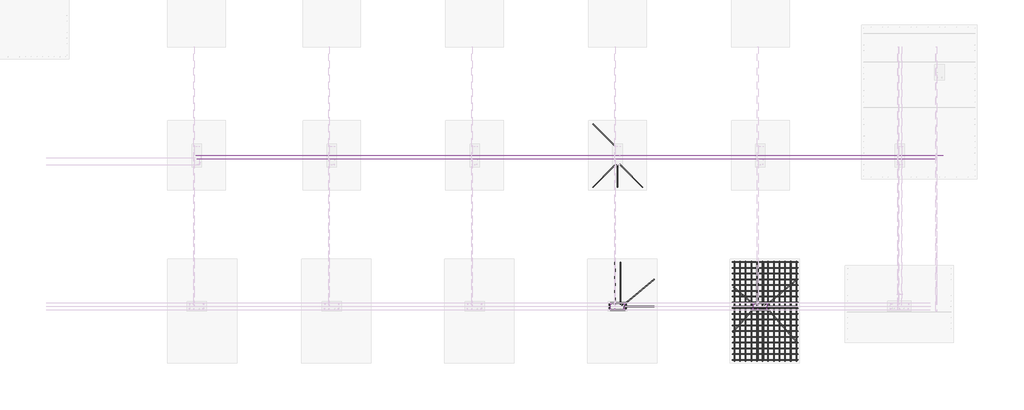
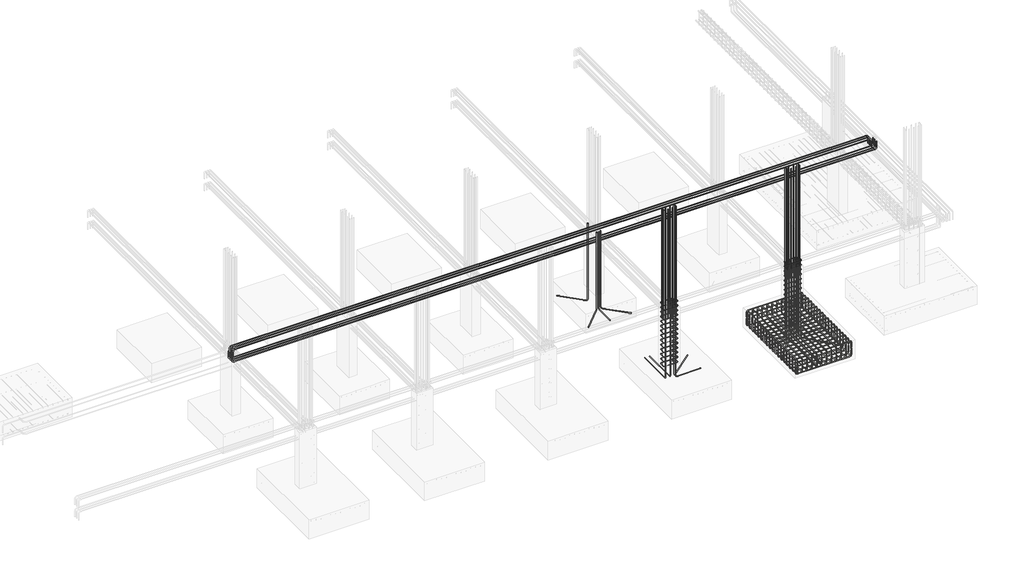
# One storey, part 7 of 18: 39 reinforcing bars.
"""IFC4 building model written with IfcOpenShell, lengths in millimetres."""

from ifc_helpers import new_model, si_unit, point, frame, origin, place, context, project, spatial, polyline, circle_curve, trimmed, segment, composite_curve, source, transform, mapped, element, save
from ifc_brep_helpers import swept_disk

model = new_model("IFC4")

# Units and contexts
model_context = context("Model", 3, world=origin())
ifc_project = project(units=[si_unit("LENGTHUNIT", "METRE", prefix="MILLI")], contexts=[model_context])

# Site, building, storey
site = spatial("IfcSite", under=ifc_project)
building = spatial("IfcBuilding", under=site)
storey = spatial("IfcBuildingStorey", under=building, Elevation=-2000.0)

# Reinforcing bars
placement = place(None, origin())
reinforcing_bar_shape = source(origin(), model_context, "Body", "SolidModel", [
    swept_disk(composite_curve([segment(polyline([(6891.7059943, -4415.5752408, -2300.0), (6891.7059943, -4415.5752408, -2486.6)]), True, "CONTINUOUS"), segment(trimmed(circle_curve(frame((6836.2559943, -4415.5752408, -2486.6), z_axis=(0.0, 1.0, 0.0), x_axis=(55.45000000000073, 0.0, 0.0)), 55.45), [point((6891.7059943, -4415.5752408, -2486.6))], [point((6836.2559943, -4415.5752408, -2542.05))], True, "CARTESIAN"), True, "CONTINUOUS"), segment(polyline([(6836.2559943, -4415.5752408, -2542.05), (5263.0559943, -4415.5752408, -2542.05)]), True, "CONTINUOUS"), segment(trimmed(circle_curve(frame((5263.0559943, -4415.5752408, -2486.6), z_axis=(0.0, 1.0, 0.0), x_axis=(0.0, 0.0, -55.45000000000027)), 55.45), [point((5263.0559943, -4415.5752408, -2542.05))], [point((5207.6059943, -4415.5752408, -2486.6))], True, "CARTESIAN"), True, "CONTINUOUS"), segment(polyline([(5207.6059943, -4415.5752408, -2486.6), (5207.6059943, -4415.5752408, -2300.0)]), True, "CONTINUOUS")], self_intersect=False), 7.95),
])
element("IfcReinforcingBar", 1, at=placement, inside=storey, context=model_context, shape_type="MappedRepresentation", body=[
    mapped(reinforcing_bar_shape, transform((0.0, 0.0, 0.0), x_axis=(1.0, 0.0, 0.0), y_axis=(0.0, 1.0, 0.0), z_axis=(0.0, 0.0, 1.0))),
    mapped(reinforcing_bar_shape, transform((0.0, -148.9809282, 0.0), x_axis=(1.0, 0.0, 0.0), y_axis=(0.0, 1.0, 0.0), z_axis=(0.0, 0.0, 1.0))),
    mapped(reinforcing_bar_shape, transform((0.0, -297.9618564, 0.0), x_axis=(1.0, 0.0, 0.0), y_axis=(0.0, 1.0, 0.0), z_axis=(0.0, 0.0, 1.0))),
    mapped(reinforcing_bar_shape, transform((0.0, -446.9427846, 0.0), x_axis=(1.0, 0.0, 0.0), y_axis=(0.0, 1.0, 0.0), z_axis=(0.0, 0.0, 1.0))),
    mapped(reinforcing_bar_shape, transform((0.0, -595.9237129, 0.0), x_axis=(1.0, 0.0, 0.0), y_axis=(0.0, 1.0, 0.0), z_axis=(0.0, 0.0, 1.0))),
    mapped(reinforcing_bar_shape, transform((0.0, -744.9046411, 0.0), x_axis=(1.0, 0.0, 0.0), y_axis=(0.0, 1.0, 0.0), z_axis=(0.0, 0.0, 1.0))),
    mapped(reinforcing_bar_shape, transform((0.0, -893.8855693, 0.0), x_axis=(1.0, 0.0, 0.0), y_axis=(0.0, 1.0, 0.0), z_axis=(0.0, 0.0, 1.0))),
    mapped(reinforcing_bar_shape, transform((0.0, -1042.8664975, 0.0), x_axis=(1.0, 0.0, 0.0), y_axis=(0.0, 1.0, 0.0), z_axis=(0.0, 0.0, 1.0))),
    mapped(reinforcing_bar_shape, transform((0.0, -1191.8474257, 0.0), x_axis=(1.0, 0.0, 0.0), y_axis=(0.0, 1.0, 0.0), z_axis=(0.0, 0.0, 1.0))),
    mapped(reinforcing_bar_shape, transform((0.0, -1340.8283539, 0.0), x_axis=(1.0, 0.0, 0.0), y_axis=(0.0, 1.0, 0.0), z_axis=(0.0, 0.0, 1.0))),
    mapped(reinforcing_bar_shape, transform((0.0, -1489.8092821, 0.0), x_axis=(1.0, 0.0, 0.0), y_axis=(0.0, 1.0, 0.0), z_axis=(0.0, 0.0, 1.0))),
    mapped(reinforcing_bar_shape, transform((0.0, -1638.7902103, 0.0), x_axis=(1.0, 0.0, 0.0), y_axis=(0.0, 1.0, 0.0), z_axis=(0.0, 0.0, 1.0))),
    mapped(reinforcing_bar_shape, transform((0.0, -1787.7711386, 0.0), x_axis=(1.0, 0.0, 0.0), y_axis=(0.0, 1.0, 0.0), z_axis=(0.0, 0.0, 1.0))),
    mapped(reinforcing_bar_shape, transform((0.0, -1936.7520668, 0.0), x_axis=(1.0, 0.0, 0.0), y_axis=(0.0, 1.0, 0.0), z_axis=(0.0, 0.0, 1.0))),
    mapped(reinforcing_bar_shape, transform((0.0, -2085.732995, 0.0), x_axis=(1.0, 0.0, 0.0), y_axis=(0.0, 1.0, 0.0), z_axis=(0.0, 0.0, 1.0))),
    mapped(reinforcing_bar_shape, transform((0.0, -2234.7139232, 0.0), x_axis=(1.0, 0.0, 0.0), y_axis=(0.0, 1.0, 0.0), z_axis=(0.0, 0.0, 1.0))),
    mapped(reinforcing_bar_shape, transform((0.0, -2383.6948514, 0.0), x_axis=(1.0, 0.0, 0.0), y_axis=(0.0, 1.0, 0.0), z_axis=(0.0, 0.0, 1.0))),
    mapped(reinforcing_bar_shape, transform((0.0, -2532.6757796, 0.0), x_axis=(1.0, 0.0, 0.0), y_axis=(0.0, 1.0, 0.0), z_axis=(0.0, 0.0, 1.0))),
])
reinforcing_bar_2_shape = source(origin(), model_context, "Body", "SolidModel", [
    swept_disk(composite_curve([segment(polyline([(5205.6559943, -4415.5752408, -2250.0), (5205.6559943, -4415.5752408, -2102.0)]), True, "CONTINUOUS"), segment(trimmed(circle_curve(frame((5251.6559943, -4415.5752408, -2102.0), z_axis=(0.0, 1.0, 0.0), x_axis=(-46.0, 0.0, 0.0)), 46.0), [point((5205.6559943, -4415.5752408, -2102.0))], [point((5251.6559943, -4415.5752408, -2056.0))], True, "CARTESIAN"), True, "CONTINUOUS"), segment(polyline([(5251.6559943, -4415.5752408, -2056.0), (6847.6559943, -4415.5752408, -2056.0)]), True, "CONTINUOUS"), segment(trimmed(circle_curve(frame((6847.6559943, -4415.5752408, -2102.0), z_axis=(0.0, 1.0, 0.0), x_axis=(0.0, 0.0, 46.0)), 46.0), [point((6847.6559943, -4415.5752408, -2056.0))], [point((6893.6559943, -4415.5752408, -2102.0))], True, "CARTESIAN"), True, "CONTINUOUS"), segment(polyline([(6893.6559943, -4415.5752408, -2102.0), (6893.6559943, -4415.5752408, -2250.0)]), True, "CONTINUOUS")], self_intersect=False), 6.0),
])
element("IfcReinforcingBar", 2, at=placement, inside=storey, context=model_context, shape_type="MappedRepresentation", body=[
    mapped(reinforcing_bar_2_shape, transform((0.0, 0.0, 0.0), x_axis=(1.0, 0.0, 0.0), y_axis=(0.0, 1.0, 0.0), z_axis=(0.0, 0.0, 1.0))),
    mapped(reinforcing_bar_2_shape, transform((0.0, -148.9809282, 0.0), x_axis=(1.0, 0.0, 0.0), y_axis=(0.0, 1.0, 0.0), z_axis=(0.0, 0.0, 1.0))),
    mapped(reinforcing_bar_2_shape, transform((0.0, -297.9618564, 0.0), x_axis=(1.0, 0.0, 0.0), y_axis=(0.0, 1.0, 0.0), z_axis=(0.0, 0.0, 1.0))),
    mapped(reinforcing_bar_2_shape, transform((0.0, -446.9427846, 0.0), x_axis=(1.0, 0.0, 0.0), y_axis=(0.0, 1.0, 0.0), z_axis=(0.0, 0.0, 1.0))),
    mapped(reinforcing_bar_2_shape, transform((0.0, -595.9237129, 0.0), x_axis=(1.0, 0.0, 0.0), y_axis=(0.0, 1.0, 0.0), z_axis=(0.0, 0.0, 1.0))),
    mapped(reinforcing_bar_2_shape, transform((0.0, -744.9046411, 0.0), x_axis=(1.0, 0.0, 0.0), y_axis=(0.0, 1.0, 0.0), z_axis=(0.0, 0.0, 1.0))),
    mapped(reinforcing_bar_2_shape, transform((0.0, -893.8855693, 0.0), x_axis=(1.0, 0.0, 0.0), y_axis=(0.0, 1.0, 0.0), z_axis=(0.0, 0.0, 1.0))),
    mapped(reinforcing_bar_2_shape, transform((0.0, -1042.8664975, 0.0), x_axis=(1.0, 0.0, 0.0), y_axis=(0.0, 1.0, 0.0), z_axis=(0.0, 0.0, 1.0))),
    mapped(reinforcing_bar_2_shape, transform((0.0, -1191.8474257, 0.0), x_axis=(1.0, 0.0, 0.0), y_axis=(0.0, 1.0, 0.0), z_axis=(0.0, 0.0, 1.0))),
    mapped(reinforcing_bar_2_shape, transform((0.0, -1340.8283539, 0.0), x_axis=(1.0, 0.0, 0.0), y_axis=(0.0, 1.0, 0.0), z_axis=(0.0, 0.0, 1.0))),
    mapped(reinforcing_bar_2_shape, transform((0.0, -1489.8092821, 0.0), x_axis=(1.0, 0.0, 0.0), y_axis=(0.0, 1.0, 0.0), z_axis=(0.0, 0.0, 1.0))),
    mapped(reinforcing_bar_2_shape, transform((0.0, -1638.7902103, 0.0), x_axis=(1.0, 0.0, 0.0), y_axis=(0.0, 1.0, 0.0), z_axis=(0.0, 0.0, 1.0))),
    mapped(reinforcing_bar_2_shape, transform((0.0, -1787.7711386, 0.0), x_axis=(1.0, 0.0, 0.0), y_axis=(0.0, 1.0, 0.0), z_axis=(0.0, 0.0, 1.0))),
    mapped(reinforcing_bar_2_shape, transform((0.0, -1936.7520668, 0.0), x_axis=(1.0, 0.0, 0.0), y_axis=(0.0, 1.0, 0.0), z_axis=(0.0, 0.0, 1.0))),
    mapped(reinforcing_bar_2_shape, transform((0.0, -2085.732995, 0.0), x_axis=(1.0, 0.0, 0.0), y_axis=(0.0, 1.0, 0.0), z_axis=(0.0, 0.0, 1.0))),
    mapped(reinforcing_bar_2_shape, transform((0.0, -2234.7139232, 0.0), x_axis=(1.0, 0.0, 0.0), y_axis=(0.0, 1.0, 0.0), z_axis=(0.0, 0.0, 1.0))),
    mapped(reinforcing_bar_2_shape, transform((0.0, -2383.6948514, 0.0), x_axis=(1.0, 0.0, 0.0), y_axis=(0.0, 1.0, 0.0), z_axis=(0.0, 0.0, 1.0))),
    mapped(reinforcing_bar_2_shape, transform((0.0, -2532.6757796, 0.0), x_axis=(1.0, 0.0, 0.0), y_axis=(0.0, 1.0, 0.0), z_axis=(0.0, 0.0, 1.0))),
])
reinforcing_bar_3_shape = source(origin(), model_context, "Body", "SolidModel", [
    swept_disk(composite_curve([segment(polyline([(5251.8367771, -4392.6797656, -2322.6684255), (5251.8367771, -4392.6797656, -2470.6684255)]), True, "CONTINUOUS"), segment(trimmed(circle_curve(frame((5251.8367771, -4438.6797656, -2470.6684255), z_axis=(-1.0, 0.0, 0.0), x_axis=(0.0, 46.0, 0.0)), 46.0), [point((5251.8367771, -4392.6797656, -2470.6684255))], [point((5251.8367771, -4438.6797656, -2516.6684255))], True, "CARTESIAN"), True, "CONTINUOUS"), segment(polyline([(5251.8367771, -4438.6797656, -2516.6684255), (5251.8367771, -6934.6797656, -2516.6684255)]), True, "CONTINUOUS"), segment(trimmed(circle_curve(frame((5251.8367771, -6934.6797656, -2470.6684255), z_axis=(-1.0, 0.0, 0.0), x_axis=(0.0, 0.0, -46.0)), 46.0), [point((5251.8367771, -6934.6797656, -2516.6684255))], [point((5251.8367771, -6980.6797656, -2470.6684255))], True, "CARTESIAN"), True, "CONTINUOUS"), segment(polyline([(5251.8367771, -6980.6797656, -2470.6684255), (5251.8367771, -6980.6797656, -2322.6684255)]), True, "CONTINUOUS")], self_intersect=False), 6.0),
])
element("IfcReinforcingBar", 3, at=placement, inside=storey, context=model_context, shape_type="MappedRepresentation", body=[
    mapped(reinforcing_bar_3_shape, transform((0.0, 0.0, 0.0), x_axis=(1.0, 0.0, 0.0), y_axis=(0.0, 1.0, 0.0), z_axis=(0.0, 0.0, 1.0))),
    mapped(reinforcing_bar_3_shape, transform((145.8017329, 0.0, 0.0), x_axis=(1.0, 0.0, 0.0), y_axis=(0.0, 1.0, 0.0), z_axis=(0.0, 0.0, 1.0))),
    mapped(reinforcing_bar_3_shape, transform((291.6034659, 0.0, 0.0), x_axis=(1.0, 0.0, 0.0), y_axis=(0.0, 1.0, 0.0), z_axis=(0.0, 0.0, 1.0))),
    mapped(reinforcing_bar_3_shape, transform((437.4051988, 0.0, 0.0), x_axis=(1.0, 0.0, 0.0), y_axis=(0.0, 1.0, 0.0), z_axis=(0.0, 0.0, 1.0))),
    mapped(reinforcing_bar_3_shape, transform((583.2069318, 0.0, 0.0), x_axis=(1.0, 0.0, 0.0), y_axis=(0.0, 1.0, 0.0), z_axis=(0.0, 0.0, 1.0))),
    mapped(reinforcing_bar_3_shape, transform((729.0086647, 0.0, 0.0), x_axis=(1.0, 0.0, 0.0), y_axis=(0.0, 1.0, 0.0), z_axis=(0.0, 0.0, 1.0))),
    mapped(reinforcing_bar_3_shape, transform((874.8103976, 0.0, 0.0), x_axis=(1.0, 0.0, 0.0), y_axis=(0.0, 1.0, 0.0), z_axis=(0.0, 0.0, 1.0))),
    mapped(reinforcing_bar_3_shape, transform((1020.6121306, 0.0, 0.0), x_axis=(1.0, 0.0, 0.0), y_axis=(0.0, 1.0, 0.0), z_axis=(0.0, 0.0, 1.0))),
    mapped(reinforcing_bar_3_shape, transform((1166.4138635, 0.0, 0.0), x_axis=(1.0, 0.0, 0.0), y_axis=(0.0, 1.0, 0.0), z_axis=(0.0, 0.0, 1.0))),
    mapped(reinforcing_bar_3_shape, transform((1312.2155965, 0.0, 0.0), x_axis=(1.0, 0.0, 0.0), y_axis=(0.0, 1.0, 0.0), z_axis=(0.0, 0.0, 1.0))),
    mapped(reinforcing_bar_3_shape, transform((1458.0173294, 0.0, 0.0), x_axis=(1.0, 0.0, 0.0), y_axis=(0.0, 1.0, 0.0), z_axis=(0.0, 0.0, 1.0))),
    mapped(reinforcing_bar_3_shape, transform((1603.8190623, 0.0, 0.0), x_axis=(1.0, 0.0, 0.0), y_axis=(0.0, 1.0, 0.0), z_axis=(0.0, 0.0, 1.0))),
])
reinforcing_bar_4_shape = source(origin(), model_context, "Body", "SolidModel", [
    swept_disk(composite_curve([segment(polyline([(6857.5790113, -4392.6797656, -2276.6677805), (6857.5790113, -4392.6797656, -2128.6677805)]), True, "CONTINUOUS"), segment(trimmed(circle_curve(frame((6857.5790113, -4438.6797656, -2128.6677805), z_axis=(1.0, 0.0, 0.0), x_axis=(0.0, 46.0, 0.0)), 46.0), [point((6857.5790113, -4392.6797656, -2128.6677805))], [point((6857.5790113, -4438.6797656, -2082.6677805))], True, "CARTESIAN"), True, "CONTINUOUS"), segment(polyline([(6857.5790113, -4438.6797656, -2082.6677805), (6857.5790113, -6934.6797656, -2082.6677805)]), True, "CONTINUOUS"), segment(trimmed(circle_curve(frame((6857.5790113, -6934.6797656, -2128.6677805), z_axis=(1.0, 0.0, 0.0), x_axis=(0.0, 0.0, 46.0)), 46.0), [point((6857.5790113, -6934.6797656, -2082.6677805))], [point((6857.5790113, -6980.6797656, -2128.6677805))], True, "CARTESIAN"), True, "CONTINUOUS"), segment(polyline([(6857.5790113, -6980.6797656, -2128.6677805), (6857.5790113, -6980.6797656, -2276.6677805)]), True, "CONTINUOUS")], self_intersect=False), 6.0),
])
element("IfcReinforcingBar", 4, at=placement, inside=storey, context=model_context, shape_type="MappedRepresentation", body=[
    mapped(reinforcing_bar_4_shape, transform((0.0, 0.0, 0.0), x_axis=(1.0, 0.0, 0.0), y_axis=(0.0, 1.0, 0.0), z_axis=(0.0, 0.0, 1.0))),
    mapped(reinforcing_bar_4_shape, transform((-145.9765667, 0.0, 0.0), x_axis=(1.0, 0.0, 0.0), y_axis=(0.0, 1.0, 0.0), z_axis=(0.0, 0.0, 1.0))),
    mapped(reinforcing_bar_4_shape, transform((-291.9531335, 0.0, 0.0), x_axis=(1.0, 0.0, 0.0), y_axis=(0.0, 1.0, 0.0), z_axis=(0.0, 0.0, 1.0))),
    mapped(reinforcing_bar_4_shape, transform((-437.9297002, 0.0, 0.0), x_axis=(1.0, 0.0, 0.0), y_axis=(0.0, 1.0, 0.0), z_axis=(0.0, 0.0, 1.0))),
    mapped(reinforcing_bar_4_shape, transform((-583.906267, 0.0, 0.0), x_axis=(1.0, 0.0, 0.0), y_axis=(0.0, 1.0, 0.0), z_axis=(0.0, 0.0, 1.0))),
    mapped(reinforcing_bar_4_shape, transform((-729.8828337, 0.0, 0.0), x_axis=(1.0, 0.0, 0.0), y_axis=(0.0, 1.0, 0.0), z_axis=(0.0, 0.0, 1.0))),
    mapped(reinforcing_bar_4_shape, transform((-875.8594005, 0.0, 0.0), x_axis=(1.0, 0.0, 0.0), y_axis=(0.0, 1.0, 0.0), z_axis=(0.0, 0.0, 1.0))),
    mapped(reinforcing_bar_4_shape, transform((-1021.8359672, 0.0, 0.0), x_axis=(1.0, 0.0, 0.0), y_axis=(0.0, 1.0, 0.0), z_axis=(0.0, 0.0, 1.0))),
    mapped(reinforcing_bar_4_shape, transform((-1167.8125339, 0.0, 0.0), x_axis=(1.0, 0.0, 0.0), y_axis=(0.0, 1.0, 0.0), z_axis=(0.0, 0.0, 1.0))),
    mapped(reinforcing_bar_4_shape, transform((-1313.7891007, 0.0, 0.0), x_axis=(1.0, 0.0, 0.0), y_axis=(0.0, 1.0, 0.0), z_axis=(0.0, 0.0, 1.0))),
    mapped(reinforcing_bar_4_shape, transform((-1459.7656674, 0.0, 0.0), x_axis=(1.0, 0.0, 0.0), y_axis=(0.0, 1.0, 0.0), z_axis=(0.0, 0.0, 1.0))),
    mapped(reinforcing_bar_4_shape, transform((-1605.7422342, 0.0, 0.0), x_axis=(1.0, 0.0, 0.0), y_axis=(0.0, 1.0, 0.0), z_axis=(0.0, 0.0, 1.0))),
])
reinforcing_bar_5_shape = source(origin(), model_context, "Body", "SolidModel", [
    swept_disk(composite_curve([segment(polyline([(6039.5684825, -5535.5091206, -34.0), (6095.9039341, -5479.1736689, -34.0)]), True, "CONTINUOUS"), segment(trimmed(circle_curve(frame((6116.4100308, -5499.6797656, -34.0), z_axis=(0.0, 0.0, -1.0), x_axis=(-20.506096699999944, 20.506096699999944, 0.0)), 29.0), [point((6095.9039341, -5479.1736689, -34.0))], [point((6145.4100308, -5499.6797656, -34.0))], True, "CARTESIAN"), True, "CONTINUOUS"), segment(polyline([(6145.4100308, -5499.6797656, -34.0), (6145.4100308, -5623.6797656, -34.0)]), True, "CONTINUOUS"), segment(trimmed(circle_curve(frame((6116.4100308, -5623.6797656, -34.0), z_axis=(0.0, 0.0, -1.0), x_axis=(29.0, 0.0, 0.0)), 29.0), [point((6145.4100308, -5623.6797656, -34.0))], [point((6116.4100308, -5652.6797656, -34.0))], True, "CARTESIAN"), True, "CONTINUOUS"), segment(polyline([(6116.4100308, -5652.6797656, -34.0), (5742.4100308, -5652.6797656, -34.0)]), True, "CONTINUOUS"), segment(trimmed(circle_curve(frame((5742.4100308, -5623.707741, -32.7265044), z_axis=(0.0, 0.043913640913297095, -0.9990353307775146), x_axis=(0.0, -28.972024599999713, -1.2734955999999968)), 29.0), [point((5742.4100308, -5652.6797656, -34.0))], [point((5713.4100308, -5623.707741, -32.7265044))], True, "CARTESIAN"), True, "CONTINUOUS"), segment(polyline([(5713.4100308, -5623.707741, -32.7265044), (5713.4100308, -5499.6517902, -27.2734956)]), True, "CONTINUOUS"), segment(trimmed(circle_curve(frame((5742.4100308, -5499.6517902, -27.2734956), z_axis=(0.0, 0.043913640913297095, -0.9990353307775146), x_axis=(-29.0, 0.0, 0.0)), 29.0), [point((5713.4100308, -5499.6517902, -27.2734956))], [point((5742.4100308, -5470.6797656, -26.0))], True, "CARTESIAN"), True, "CONTINUOUS"), segment(polyline([(5742.4100308, -5470.6797656, -26.0), (6116.4100308, -5470.6797656, -26.0)]), True, "CONTINUOUS"), segment(trimmed(circle_curve(frame((6116.4100308, -5499.6797656, -26.0), z_axis=(0.0, 0.0, -1.0), x_axis=(0.0, 29.0, 0.0)), 29.0), [point((6116.4100308, -5470.6797656, -26.0))], [point((6136.9161274, -5520.1858622, -26.0))], True, "CARTESIAN"), True, "CONTINUOUS"), segment(polyline([(6136.9161274, -5520.1858622, -26.0), (6080.5806758, -5576.5213139, -26.0)]), True, "CONTINUOUS")], self_intersect=False), 4.0),
])
element("IfcReinforcingBar", 5, at=placement, inside=storey, context=model_context, shape_type="MappedRepresentation", body=[
    mapped(reinforcing_bar_5_shape, transform((0.0, 0.0, 0.0), x_axis=(1.0, 0.0, 0.0), y_axis=(0.0, 1.0, 0.0), z_axis=(0.0, 0.0, 1.0))),
    mapped(reinforcing_bar_5_shape, transform((0.0, 0.0, -148.6153846), x_axis=(1.0, 0.0, 0.0), y_axis=(0.0, 1.0, 0.0), z_axis=(0.0, 0.0, 1.0))),
    mapped(reinforcing_bar_5_shape, transform((0.0, 0.0, -297.2307692), x_axis=(1.0, 0.0, 0.0), y_axis=(0.0, 1.0, 0.0), z_axis=(0.0, 0.0, 1.0))),
    mapped(reinforcing_bar_5_shape, transform((0.0, 0.0, -445.8461538), x_axis=(1.0, 0.0, 0.0), y_axis=(0.0, 1.0, 0.0), z_axis=(0.0, 0.0, 1.0))),
    mapped(reinforcing_bar_5_shape, transform((0.0, 0.0, -594.4615385), x_axis=(1.0, 0.0, 0.0), y_axis=(0.0, 1.0, 0.0), z_axis=(0.0, 0.0, 1.0))),
    mapped(reinforcing_bar_5_shape, transform((0.0, 0.0, -743.0769231), x_axis=(1.0, 0.0, 0.0), y_axis=(0.0, 1.0, 0.0), z_axis=(0.0, 0.0, 1.0))),
    mapped(reinforcing_bar_5_shape, transform((0.0, 0.0, -891.6923077), x_axis=(1.0, 0.0, 0.0), y_axis=(0.0, 1.0, 0.0), z_axis=(0.0, 0.0, 1.0))),
    mapped(reinforcing_bar_5_shape, transform((0.0, 0.0, -1040.3076923), x_axis=(1.0, 0.0, 0.0), y_axis=(0.0, 1.0, 0.0), z_axis=(0.0, 0.0, 1.0))),
    mapped(reinforcing_bar_5_shape, transform((0.0, 0.0, -1188.9230769), x_axis=(1.0, 0.0, 0.0), y_axis=(0.0, 1.0, 0.0), z_axis=(0.0, 0.0, 1.0))),
    mapped(reinforcing_bar_5_shape, transform((0.0, 0.0, -1337.5384615), x_axis=(1.0, 0.0, 0.0), y_axis=(0.0, 1.0, 0.0), z_axis=(0.0, 0.0, 1.0))),
    mapped(reinforcing_bar_5_shape, transform((0.0, 0.0, -1486.1538462), x_axis=(1.0, 0.0, 0.0), y_axis=(0.0, 1.0, 0.0), z_axis=(0.0, 0.0, 1.0))),
    mapped(reinforcing_bar_5_shape, transform((0.0, 0.0, -1634.7692308), x_axis=(1.0, 0.0, 0.0), y_axis=(0.0, 1.0, 0.0), z_axis=(0.0, 0.0, 1.0))),
    mapped(reinforcing_bar_5_shape, transform((0.0, 0.0, -1783.3846154), x_axis=(1.0, 0.0, 0.0), y_axis=(0.0, 1.0, 0.0), z_axis=(0.0, 0.0, 1.0))),
    mapped(reinforcing_bar_5_shape, transform((0.0, 0.0, -1932.0), x_axis=(1.0, 0.0, 0.0), y_axis=(0.0, 1.0, 0.0), z_axis=(0.0, 0.0, 1.0))),
])
element("IfcReinforcingBar", 6, at=placement, inside=storey, context=model_context, shape_type="SolidModel", body=[
    swept_disk(composite_curve([segment(polyline([(5226.3766571, -5063.6864072, -2480.0), (5699.5441951, -5460.7211138, -2480.0)]), True, "CONTINUOUS"), segment(trimmed(circle_curve(frame((5699.5441951, -5460.7211138, -2412.5), z_axis=(-0.6427876096865429, -0.7660444431189751, 0.0), x_axis=(0.0, 0.0, -67.5)), 67.5), [point((5699.5441951, -5460.7211138, -2480.0))], [point((5751.252195, -5504.1092774, -2412.5))], True, "CARTESIAN"), True, "CONTINUOUS"), segment(polyline([(5751.252195, -5504.1092774, -2412.5), (5751.252195, -5504.1092774, -20.0)]), True, "CONTINUOUS")], self_intersect=False), 10.0),
])
element("IfcReinforcingBar", 7, at=placement, inside=storey, context=model_context, shape_type="SolidModel", body=[
    swept_disk(composite_curve([segment(polyline([(5222.3423379, -5559.3632831, -2480.0), (5694.892069, -5559.3632831, -2480.0)]), True, "CONTINUOUS"), segment(trimmed(circle_curve(frame((5694.892069, -5559.3632831, -2434.0), z_axis=(0.0, -1.0, 0.0), x_axis=(0.0, 0.0, -46.0)), 46.0), [point((5694.892069, -5559.3632831, -2480.0))], [point((5740.892069, -5559.3632831, -2434.0))], True, "CARTESIAN"), True, "CONTINUOUS"), segment(polyline([(5740.892069, -5559.3632831, -2434.0), (5740.892069, -5559.3632831, -30.0)]), True, "CONTINUOUS")], self_intersect=False), 6.0),
])
element("IfcReinforcingBar", 8, at=placement, inside=storey, context=model_context, shape_type="SolidModel", body=[
    swept_disk(composite_curve([segment(polyline([(6872.9353315, -4861.8897199, -2480.0), (6159.2758664, -5460.7211138, -2480.0)]), True, "CONTINUOUS"), segment(trimmed(circle_curve(frame((6159.2758664, -5460.7211138, -2412.5), z_axis=(-0.6427876096865429, 0.7660444431189751, 0.0), x_axis=(0.0, 0.0, -67.5)), 67.5), [point((6159.2758664, -5460.7211138, -2480.0))], [point((6107.5678665, -5504.1092774, -2412.5))], True, "CARTESIAN"), True, "CONTINUOUS"), segment(polyline([(6107.5678665, -5504.1092774, -2412.5), (6107.5678665, -5504.1092774, -20.0)]), True, "CONTINUOUS")], self_intersect=False), 10.0),
])
element("IfcReinforcingBar", 9, at=placement, inside=storey, context=model_context, shape_type="SolidModel", body=[
    swept_disk(composite_curve([segment(polyline([(5219.3758106, -6231.1040429, -2480.0), (5706.9682106, -5670.1931504, -2480.0)]), True, "CONTINUOUS"), segment(trimmed(circle_curve(frame((5706.9682106, -5670.1931504, -2412.5), z_axis=(0.7547095802227678, -0.6560590289905122, 0.0), x_axis=(0.0, 0.0, -67.5)), 67.5), [point((5706.9682106, -5670.1931504, -2480.0))], [point((5751.252195, -5619.2502537, -2412.5))], True, "CARTESIAN"), True, "CONTINUOUS"), segment(polyline([(5751.252195, -5619.2502537, -2412.5), (5751.252195, -5619.2502537, -20.0)]), True, "CONTINUOUS")], self_intersect=False), 10.0),
])
element("IfcReinforcingBar", 10, at=placement, inside=storey, context=model_context, shape_type="SolidModel", body=[
    swept_disk(composite_curve([segment(polyline([(6879.936178, -6507.7583579, -2480.0), (6151.851851, -5670.1931504, -2480.0)]), True, "CONTINUOUS"), segment(trimmed(circle_curve(frame((6151.851851, -5670.1931504, -2412.5), z_axis=(0.7547095802227678, 0.6560590289905122, 0.0), x_axis=(0.0, 0.0, -67.5)), 67.5), [point((6151.851851, -5670.1931504, -2480.0))], [point((6107.5678665, -5619.2502537, -2412.5))], True, "CARTESIAN"), True, "CONTINUOUS"), segment(polyline([(6107.5678665, -5619.2502537, -2412.5), (6107.5678665, -5619.2502537, -20.0)]), True, "CONTINUOUS")], self_intersect=False), 10.0),
])
element("IfcReinforcingBar", 11, at=placement, inside=storey, context=model_context, shape_type="SolidModel", body=[
    swept_disk(composite_curve([segment(polyline([(6876.9696507, -5559.3632831, -2480.0), (6163.9279926, -5559.3632831, -2480.0)]), True, "CONTINUOUS"), segment(trimmed(circle_curve(frame((6163.9279926, -5559.3632831, -2434.0), z_axis=(0.0, 1.0, 0.0), x_axis=(0.0, 0.0, -46.0)), 46.0), [point((6163.9279926, -5559.3632831, -2480.0))], [point((6117.9279926, -5559.3632831, -2434.0))], True, "CARTESIAN"), True, "CONTINUOUS"), segment(polyline([(6117.9279926, -5559.3632831, -2434.0), (6117.9279926, -5559.3632831, -30.0)]), True, "CONTINUOUS")], self_intersect=False), 6.0),
])
reinforcing_bar_6_shape = source(origin(), model_context, "Body", "SolidModel", [
    swept_disk(composite_curve([segment(polyline([(5856.3579357, -6948.2510204, -2480.0), (5856.3579357, -5673.717598, -2480.0)]), True, "CONTINUOUS"), segment(trimmed(circle_curve(frame((5856.3579357, -5673.717598, -2434.0), z_axis=(1.0, 0.0, 0.0), x_axis=(0.0, 0.0, -46.0)), 46.0), [point((5856.3579357, -5673.717598, -2480.0))], [point((5856.3579357, -5627.717598, -2434.0))], True, "CARTESIAN"), True, "CONTINUOUS"), segment(polyline([(5856.3579357, -5627.717598, -2434.0), (5856.3579357, -5627.717598, -30.0)]), True, "CONTINUOUS")], self_intersect=False), 6.0),
])
element("IfcReinforcingBar", 12, at=placement, inside=storey, context=model_context, shape_type="MappedRepresentation", body=[
    mapped(reinforcing_bar_6_shape, transform((0.0, 0.0, 0.0), x_axis=(1.0, 0.0, 0.0), y_axis=(0.0, 1.0, 0.0), z_axis=(0.0, 0.0, 1.0))),
    mapped(reinforcing_bar_6_shape, transform((144.9594019, 0.0, 0.0), x_axis=(1.0, 0.0, 0.0), y_axis=(0.0, 1.0, 0.0), z_axis=(0.0, 0.0, 1.0))),
])
reinforcing_bar_7_shape = source(origin(), model_context, "Body", "SolidModel", [
    swept_disk(composite_curve([segment(polyline([(5856.3579357, -4416.634351, -2480.0), (5856.3579357, -5449.6419331, -2480.0)]), True, "CONTINUOUS"), segment(trimmed(circle_curve(frame((5856.3579357, -5449.6419331, -2434.0), z_axis=(-1.0, 0.0, 0.0), x_axis=(0.0, 0.0, -46.0)), 46.0), [point((5856.3579357, -5449.6419331, -2480.0))], [point((5856.3579357, -5495.6419331, -2434.0))], True, "CARTESIAN"), True, "CONTINUOUS"), segment(polyline([(5856.3579357, -5495.6419331, -2434.0), (5856.3579357, -5495.6419331, -30.0)]), True, "CONTINUOUS")], self_intersect=False), 6.0),
])
element("IfcReinforcingBar", 13, at=placement, inside=storey, context=model_context, shape_type="MappedRepresentation", body=[
    mapped(reinforcing_bar_7_shape, transform((0.0, 0.0, 0.0), x_axis=(1.0, 0.0, 0.0), y_axis=(0.0, 1.0, 0.0), z_axis=(0.0, 0.0, 1.0))),
    mapped(reinforcing_bar_7_shape, transform((144.9594019, 0.0, 0.0), x_axis=(1.0, 0.0, 0.0), y_axis=(0.0, 1.0, 0.0), z_axis=(0.0, 0.0, 1.0))),
])
reinforcing_bar_8_shape = source(origin(), model_context, "Body", "SolidModel", [
    swept_disk(composite_curve([segment(polyline([(2339.5684825, -5535.5091206, -34.0), (2395.9039341, -5479.1736689, -34.0)]), True, "CONTINUOUS"), segment(trimmed(circle_curve(frame((2416.4100308, -5499.6797656, -34.0), z_axis=(0.0, 0.0, -1.0), x_axis=(-20.5060967000004, 20.506096699999944, 0.0)), 29.0), [point((2395.9039341, -5479.1736689, -34.0))], [point((2445.4100308, -5499.6797656, -34.0))], True, "CARTESIAN"), True, "CONTINUOUS"), segment(polyline([(2445.4100308, -5499.6797656, -34.0), (2445.4100308, -5623.6797656, -34.0)]), True, "CONTINUOUS"), segment(trimmed(circle_curve(frame((2416.4100308, -5623.6797656, -34.0), z_axis=(0.0, 0.0, -1.0), x_axis=(29.0, 0.0, 0.0)), 29.0), [point((2445.4100308, -5623.6797656, -34.0))], [point((2416.4100308, -5652.6797656, -34.0))], True, "CARTESIAN"), True, "CONTINUOUS"), segment(polyline([(2416.4100308, -5652.6797656, -34.0), (2042.4100308, -5652.6797656, -34.0)]), True, "CONTINUOUS"), segment(trimmed(circle_curve(frame((2042.4100308, -5623.707741, -32.7265044), z_axis=(0.0, 0.043913640913297095, -0.9990353307775146), x_axis=(0.0, -28.972024599999713, -1.2734955999999968)), 29.0), [point((2042.4100308, -5652.6797656, -34.0))], [point((2013.4100308, -5623.707741, -32.7265044))], True, "CARTESIAN"), True, "CONTINUOUS"), segment(polyline([(2013.4100308, -5623.707741, -32.7265044), (2013.4100308, -5499.6517902, -27.2734956)]), True, "CONTINUOUS"), segment(trimmed(circle_curve(frame((2042.4100308, -5499.6517902, -27.2734956), z_axis=(0.0, 0.043913640913297095, -0.9990353307775146), x_axis=(-29.0, 0.0, 0.0)), 29.0), [point((2013.4100308, -5499.6517902, -27.2734956))], [point((2042.4100308, -5470.6797656, -26.0))], True, "CARTESIAN"), True, "CONTINUOUS"), segment(polyline([(2042.4100308, -5470.6797656, -26.0), (2416.4100308, -5470.6797656, -26.0)]), True, "CONTINUOUS"), segment(trimmed(circle_curve(frame((2416.4100308, -5499.6797656, -26.0), z_axis=(0.0, 0.0, -1.0), x_axis=(0.0, 29.0, 0.0)), 29.0), [point((2416.4100308, -5470.6797656, -26.0))], [point((2436.9161274, -5520.1858622, -26.0))], True, "CARTESIAN"), True, "CONTINUOUS"), segment(polyline([(2436.9161274, -5520.1858622, -26.0), (2380.5806758, -5576.5213139, -26.0)]), True, "CONTINUOUS")], self_intersect=False), 4.0),
])
element("IfcReinforcingBar", 14, at=placement, inside=storey, context=model_context, shape_type="MappedRepresentation", body=[
    mapped(reinforcing_bar_8_shape, transform((0.0, 0.0, 0.0), x_axis=(1.0, 0.0, 0.0), y_axis=(0.0, 1.0, 0.0), z_axis=(0.0, 0.0, 1.0))),
    mapped(reinforcing_bar_8_shape, transform((0.0, 0.0, -148.6153846), x_axis=(1.0, 0.0, 0.0), y_axis=(0.0, 1.0, 0.0), z_axis=(0.0, 0.0, 1.0))),
    mapped(reinforcing_bar_8_shape, transform((0.0, 0.0, -297.2307692), x_axis=(1.0, 0.0, 0.0), y_axis=(0.0, 1.0, 0.0), z_axis=(0.0, 0.0, 1.0))),
    mapped(reinforcing_bar_8_shape, transform((0.0, 0.0, -445.8461538), x_axis=(1.0, 0.0, 0.0), y_axis=(0.0, 1.0, 0.0), z_axis=(0.0, 0.0, 1.0))),
    mapped(reinforcing_bar_8_shape, transform((0.0, 0.0, -594.4615385), x_axis=(1.0, 0.0, 0.0), y_axis=(0.0, 1.0, 0.0), z_axis=(0.0, 0.0, 1.0))),
    mapped(reinforcing_bar_8_shape, transform((0.0, 0.0, -743.0769231), x_axis=(1.0, 0.0, 0.0), y_axis=(0.0, 1.0, 0.0), z_axis=(0.0, 0.0, 1.0))),
    mapped(reinforcing_bar_8_shape, transform((0.0, 0.0, -891.6923077), x_axis=(1.0, 0.0, 0.0), y_axis=(0.0, 1.0, 0.0), z_axis=(0.0, 0.0, 1.0))),
    mapped(reinforcing_bar_8_shape, transform((0.0, 0.0, -1040.3076923), x_axis=(1.0, 0.0, 0.0), y_axis=(0.0, 1.0, 0.0), z_axis=(0.0, 0.0, 1.0))),
    mapped(reinforcing_bar_8_shape, transform((0.0, 0.0, -1188.9230769), x_axis=(1.0, 0.0, 0.0), y_axis=(0.0, 1.0, 0.0), z_axis=(0.0, 0.0, 1.0))),
    mapped(reinforcing_bar_8_shape, transform((0.0, 0.0, -1337.5384615), x_axis=(1.0, 0.0, 0.0), y_axis=(0.0, 1.0, 0.0), z_axis=(0.0, 0.0, 1.0))),
    mapped(reinforcing_bar_8_shape, transform((0.0, 0.0, -1486.1538462), x_axis=(1.0, 0.0, 0.0), y_axis=(0.0, 1.0, 0.0), z_axis=(0.0, 0.0, 1.0))),
    mapped(reinforcing_bar_8_shape, transform((0.0, 0.0, -1634.7692308), x_axis=(1.0, 0.0, 0.0), y_axis=(0.0, 1.0, 0.0), z_axis=(0.0, 0.0, 1.0))),
    mapped(reinforcing_bar_8_shape, transform((0.0, 0.0, -1783.3846154), x_axis=(1.0, 0.0, 0.0), y_axis=(0.0, 1.0, 0.0), z_axis=(0.0, 0.0, 1.0))),
    mapped(reinforcing_bar_8_shape, transform((0.0, 0.0, -1932.0), x_axis=(1.0, 0.0, 0.0), y_axis=(0.0, 1.0, 0.0), z_axis=(0.0, 0.0, 1.0))),
])
element("IfcReinforcingBar", 15, at=placement, inside=storey, context=model_context, shape_type="SolidModel", body=[
    swept_disk(composite_curve([segment(polyline([(3172.9353315, -4861.8897199, -2480.0), (2459.2758664, -5460.7211138, -2480.0)]), True, "CONTINUOUS"), segment(trimmed(circle_curve(frame((2459.2758664, -5460.7211138, -2412.5), z_axis=(-0.6427876096865429, 0.7660444431189751, 0.0), x_axis=(0.0, 0.0, -67.5)), 67.5), [point((2459.2758664, -5460.7211138, -2480.0))], [point((2407.5678665, -5504.1092774, -2412.5))], True, "CARTESIAN"), True, "CONTINUOUS"), segment(polyline([(2407.5678665, -5504.1092774, -2412.5), (2407.5678665, -5504.1092774, -20.0)]), True, "CONTINUOUS")], self_intersect=False), 10.0),
])
element("IfcReinforcingBar", 16, at=placement, inside=storey, context=model_context, shape_type="SolidModel", body=[
    swept_disk(composite_curve([segment(polyline([(3176.9696507, -5559.3632831, -2480.0), (2463.9279926, -5559.3632831, -2480.0)]), True, "CONTINUOUS"), segment(trimmed(circle_curve(frame((2463.9279926, -5559.3632831, -2434.0), z_axis=(0.0, 1.0, 0.0), x_axis=(0.0, 0.0, -46.0)), 46.0), [point((2463.9279926, -5559.3632831, -2480.0))], [point((2417.9279926, -5559.3632831, -2434.0))], True, "CARTESIAN"), True, "CONTINUOUS"), segment(polyline([(2417.9279926, -5559.3632831, -2434.0), (2417.9279926, -5559.3632831, -30.0)]), True, "CONTINUOUS")], self_intersect=False), 6.0),
])
reinforcing_bar_9_shape = source(origin(), model_context, "Body", "SolidModel", [
    swept_disk(composite_curve([segment(polyline([(2156.3579357, -4416.634351, -2480.0), (2156.3579357, -5449.6419331, -2480.0)]), True, "CONTINUOUS"), segment(trimmed(circle_curve(frame((2156.3579357, -5449.6419331, -2434.0), z_axis=(-1.0, 0.0, 0.0), x_axis=(0.0, 0.0, -46.0)), 46.0), [point((2156.3579357, -5449.6419331, -2480.0))], [point((2156.3579357, -5495.6419331, -2434.0))], True, "CARTESIAN"), True, "CONTINUOUS"), segment(polyline([(2156.3579357, -5495.6419331, -2434.0), (2156.3579357, -5495.6419331, -30.0)]), True, "CONTINUOUS")], self_intersect=False), 6.0),
])
element("IfcReinforcingBar", 17, at=placement, inside=storey, context=model_context, shape_type="MappedRepresentation", body=[
    mapped(reinforcing_bar_9_shape, transform((0.0, 0.0, 0.0), x_axis=(1.0, 0.0, 0.0), y_axis=(0.0, 1.0, 0.0), z_axis=(0.0, 0.0, 1.0))),
    mapped(reinforcing_bar_9_shape, transform((144.9594019, 0.0, 0.0), x_axis=(1.0, 0.0, 0.0), y_axis=(0.0, 1.0, 0.0), z_axis=(0.0, 0.0, 1.0))),
])
element("IfcReinforcingBar", 18, at=placement, inside=storey, context=model_context, shape_type="SolidModel", body=[
    swept_disk(composite_curve([segment(polyline([(2171.6640946, -1423.0839981, -30.0), (2171.6640946, -1423.0839981, -2431.15)]), True, "CONTINUOUS"), segment(trimmed(circle_curve(frame((2132.4550236, -1383.874927, -2431.15), z_axis=(0.70710678118655, 0.707106781186545, 0.0), x_axis=(39.20907100000022, -39.209071099999846, 0.0)), 55.45), [point((2171.6640946, -1423.0839981, -2431.15))], [point((2132.4550236, -1383.874927, -2486.6))], True, "CARTESIAN"), True, "CONTINUOUS"), segment(polyline([(2132.4550236, -1383.874927, -2486.6), (1586.60971, -838.0296134, -2486.6)]), True, "CONTINUOUS")], self_intersect=False), 7.95),
])
element("IfcReinforcingBar", 19, at=placement, inside=storey, context=model_context, shape_type="SolidModel", body=[
    swept_disk(composite_curve([segment(polyline([(2228.962113, -1896.3217695, -30.0), (2228.962113, -1896.3217695, -2440.6)]), True, "CONTINUOUS"), segment(trimmed(circle_curve(frame((2228.962113, -1942.3217695, -2440.6), z_axis=(-1.0, 0.0, 0.0), x_axis=(0.0, 46.0, 0.0)), 46.0), [point((2228.962113, -1896.3217695, -2440.6))], [point((2228.962113, -1942.3217695, -2486.6))], True, "CARTESIAN"), True, "CONTINUOUS"), segment(polyline([(2228.962113, -1942.3217695, -2486.6), (2228.962113, -2479.9487164, -2486.6)]), True, "CONTINUOUS")], self_intersect=False), 6.0),
])
element("IfcReinforcingBar", 20, at=placement, inside=storey, context=model_context, shape_type="SolidModel", body=[
    swept_disk(composite_curve([segment(polyline([(2171.6640946, -1891.7202311, -30.0), (2171.6640946, -1891.7202311, -2431.15)]), True, "CONTINUOUS"), segment(trimmed(circle_curve(frame((2132.4550236, -1930.9293021, -2431.15), z_axis=(-0.7071067811865455, 0.7071067811865497, 0.0), x_axis=(39.20907100000022, 39.209070999999994, 0.0)), 55.45), [point((2171.6640946, -1891.7202311, -2431.15))], [point((2132.4550236, -1930.9293021, -2486.6))], True, "CARTESIAN"), True, "CONTINUOUS"), segment(polyline([(2132.4550236, -1930.9293021, -2486.6), (1586.60971, -2476.7746158, -2486.6)]), True, "CONTINUOUS")], self_intersect=False), 7.95),
])
element("IfcReinforcingBar", 21, at=placement, inside=storey, context=model_context, shape_type="SolidModel", body=[
    swept_disk(composite_curve([segment(polyline([(2287.1559669, -1891.7202311, -30.0), (2287.1559669, -1891.7202311, -2431.15)]), True, "CONTINUOUS"), segment(trimmed(circle_curve(frame((2326.365038, -1930.9293021, -2431.15), z_axis=(-0.7071067811865546, -0.7071067811865405, 0.0), x_axis=(-39.209071100000074, 39.209070999999994, 0.0)), 55.45), [point((2287.1559669, -1891.7202311, -2431.15))], [point((2326.365038, -1930.9293021, -2486.6))], True, "CARTESIAN"), True, "CONTINUOUS"), segment(polyline([(2326.365038, -1930.9293021, -2486.6), (2872.2103516, -2476.7746158, -2486.6)]), True, "CONTINUOUS")], self_intersect=False), 7.95),
])
reinforcing_bar_10_shape = source(origin(), model_context, "Body", "SolidModel", [
    swept_disk(composite_curve([segment(polyline([(-8649.0438073, -1567.7735095, -305.05), (-8649.0438073, -1567.7735095, -118.45)]), True, "CONTINUOUS"), segment(trimmed(circle_curve(frame((-8593.5938073, -1567.7735095, -118.45), z_axis=(0.0, 1.0, 0.0), x_axis=(-55.45000000000073, 0.0, 0.0)), 55.45), [point((-8649.0438073, -1567.7735095, -118.45))], [point((-8593.5938073, -1567.7735095, -63.0))], True, "CARTESIAN"), True, "CONTINUOUS"), segment(polyline([(-8593.5938073, -1567.7735095, -63.0), (10436.699429, -1567.7735095, -63.0)]), True, "CONTINUOUS"), segment(trimmed(circle_curve(frame((10436.699429, -1567.7735095, -118.45), z_axis=(0.0, 1.0, 0.0), x_axis=(0.0, 0.0, 55.45)), 55.45), [point((10436.699429, -1567.7735095, -63.0))], [point((10492.149429, -1567.7735095, -118.45))], True, "CARTESIAN"), True, "CONTINUOUS"), segment(polyline([(10492.149429, -1567.7735095, -118.45), (10492.149429, -1567.7735095, -305.05)]), True, "CONTINUOUS")], self_intersect=False), 7.95),
])
element("IfcReinforcingBar", 22, at=placement, inside=storey, context=model_context, shape_type="MappedRepresentation", body=[
    mapped(reinforcing_bar_10_shape, transform((0.0, 0.0, 0.0), x_axis=(1.0, 0.0, 0.0), y_axis=(0.0, 1.0, 0.0), z_axis=(0.0, 0.0, 1.0))),
    mapped(reinforcing_bar_10_shape, transform((0.0, -89.7507845, 0.0), x_axis=(1.0, 0.0, 0.0), y_axis=(0.0, 1.0, 0.0), z_axis=(0.0, 0.0, 1.0))),
    mapped(reinforcing_bar_10_shape, transform((0.0, -179.501569, 0.0), x_axis=(1.0, 0.0, 0.0), y_axis=(0.0, 1.0, 0.0), z_axis=(0.0, 0.0, 1.0))),
])
reinforcing_bar_11_shape = source(origin(), model_context, "Body", "SolidModel", [
    swept_disk(composite_curve([segment(polyline([(-8686.4025034, -1745.9711923, -197.0061706), (-8686.4025034, -1745.9711923, -383.6061706)]), True, "CONTINUOUS"), segment(trimmed(circle_curve(frame((-8630.9525034, -1745.9711923, -383.6061706), z_axis=(0.0, -1.0, 0.0), x_axis=(-55.45000000000073, 0.0, 0.0)), 55.45), [point((-8686.4025034, -1745.9711923, -383.6061706))], [point((-8630.9525034, -1745.9711923, -439.0561706))], True, "CARTESIAN"), True, "CONTINUOUS"), segment(polyline([(-8630.9525034, -1745.9711923, -439.0561706), (10587.2165048, -1745.9711923, -439.0561706)]), True, "CONTINUOUS"), segment(trimmed(circle_curve(frame((10587.2165048, -1745.9711923, -383.6061706), z_axis=(0.0, -1.0, 0.0), x_axis=(0.0, 0.0, -55.44999999999999)), 55.45), [point((10587.2165048, -1745.9711923, -439.0561706))], [point((10642.6665048, -1745.9711923, -383.6061706))], True, "CARTESIAN"), True, "CONTINUOUS"), segment(polyline([(10642.6665048, -1745.9711923, -383.6061706), (10642.6665048, -1745.9711923, -197.0061706)]), True, "CONTINUOUS")], self_intersect=False), 7.95),
])
element("IfcReinforcingBar", 23, at=placement, inside=storey, context=model_context, shape_type="MappedRepresentation", body=[
    mapped(reinforcing_bar_11_shape, transform((0.0, 0.0, 0.0), x_axis=(1.0, 0.0, 0.0), y_axis=(0.0, 1.0, 0.0), z_axis=(0.0, 0.0, 1.0))),
    mapped(reinforcing_bar_11_shape, transform((0.0, 89.8608796, 0.0), x_axis=(1.0, 0.0, 0.0), y_axis=(0.0, 1.0, 0.0), z_axis=(0.0, 0.0, 1.0))),
    mapped(reinforcing_bar_11_shape, transform((0.0, 179.7217592, 0.0), x_axis=(1.0, 0.0, 0.0), y_axis=(0.0, 1.0, 0.0), z_axis=(0.0, 0.0, 1.0))),
])
element("IfcReinforcingBar", 24, at=placement, inside=storey, context=model_context, shape_type="SolidModel", body=[
    swept_disk(composite_curve([segment(polyline([(2040.8529891, -5560.0856321, -480.0), (2040.8529891, -5560.0856321, 2970.0)]), True, "CONTINUOUS")], self_intersect=False), 6.0),
])
element("IfcReinforcingBar", 25, at=placement, inside=storey, context=model_context, shape_type="SolidModel", body=[
    swept_disk(composite_curve([segment(polyline([(2397.5287867, -5504.8316264, -480.0), (2397.5287867, -5504.8316264, 2970.0)]), True, "CONTINUOUS")], self_intersect=False), 10.0),
])
element("IfcReinforcingBar", 26, at=placement, inside=storey, context=model_context, shape_type="SolidModel", body=[
    swept_disk(composite_curve([segment(polyline([(2041.2131152, -5619.9726027, -480.0), (2041.2131152, -5619.9726027, 2970.0)]), True, "CONTINUOUS")], self_intersect=False), 10.0),
])
element("IfcReinforcingBar", 27, at=placement, inside=storey, context=model_context, shape_type="SolidModel", body=[
    swept_disk(composite_curve([segment(polyline([(2397.5287867, -5619.9726027, -480.0), (2397.5287867, -5619.9726027, 2970.0)]), True, "CONTINUOUS")], self_intersect=False), 10.0),
])
reinforcing_bar_12_shape = source(origin(), model_context, "Body", "SolidModel", [
    swept_disk(composite_curve([segment(polyline([(2146.3188559, -5627.6797656, -480.0), (2146.3188559, -5627.6797656, 2970.0)]), True, "CONTINUOUS")], self_intersect=False), 6.0),
])
element("IfcReinforcingBar", 28, at=placement, inside=storey, context=model_context, shape_type="MappedRepresentation", body=[
    mapped(reinforcing_bar_12_shape, transform((0.0, 0.0, 0.0), x_axis=(1.0, 0.0, 0.0), y_axis=(0.0, 1.0, 0.0), z_axis=(0.0, 0.0, 1.0))),
    mapped(reinforcing_bar_12_shape, transform((144.9594019, 0.0, 0.0), x_axis=(1.0, 0.0, 0.0), y_axis=(0.0, 1.0, 0.0), z_axis=(0.0, 0.0, 1.0))),
])
reinforcing_bar_13_shape = source(origin(), model_context, "Body", "SolidModel", [
    swept_disk(composite_curve([segment(polyline([(2146.3188559, -5496.3642821, -480.0), (2146.3188559, -5496.3642821, 2970.0)]), True, "CONTINUOUS")], self_intersect=False), 6.0),
])
element("IfcReinforcingBar", 29, at=placement, inside=storey, context=model_context, shape_type="MappedRepresentation", body=[
    mapped(reinforcing_bar_13_shape, transform((0.0, 0.0, 0.0), x_axis=(1.0, 0.0, 0.0), y_axis=(0.0, 1.0, 0.0), z_axis=(0.0, 0.0, 1.0))),
    mapped(reinforcing_bar_13_shape, transform((144.9594019, 0.0, 0.0), x_axis=(1.0, 0.0, 0.0), y_axis=(0.0, 1.0, 0.0), z_axis=(0.0, 0.0, 1.0))),
])
element("IfcReinforcingBar", 30, at=placement, inside=storey, context=model_context, shape_type="SolidModel", body=[
    swept_disk(composite_curve([segment(polyline([(2041.2131152, -5504.8316264, -480.0), (2041.2131152, -5504.8316264, 2970.0)]), True, "CONTINUOUS")], self_intersect=False), 10.0),
])
element("IfcReinforcingBar", 31, at=placement, inside=storey, context=model_context, shape_type="SolidModel", body=[
    swept_disk(composite_curve([segment(polyline([(2402.8889128, -5560.0856321, -480.0), (2402.8889128, -5560.0856321, 2970.0)]), True, "CONTINUOUS")], self_intersect=False), 6.0),
])
element("IfcReinforcingBar", 32, at=placement, inside=storey, context=model_context, shape_type="SolidModel", body=[
    swept_disk(composite_curve([segment(polyline([(5740.8529891, -5560.0856321, -480.0), (5740.8529891, -5560.0856321, 2970.0)]), True, "CONTINUOUS")], self_intersect=False), 6.0),
])
element("IfcReinforcingBar", 33, at=placement, inside=storey, context=model_context, shape_type="SolidModel", body=[
    swept_disk(composite_curve([segment(polyline([(6097.5287867, -5504.8316264, -480.0), (6097.5287867, -5504.8316264, 2970.0)]), True, "CONTINUOUS")], self_intersect=False), 10.0),
])
element("IfcReinforcingBar", 34, at=placement, inside=storey, context=model_context, shape_type="SolidModel", body=[
    swept_disk(composite_curve([segment(polyline([(5741.2131152, -5619.9726027, -480.0), (5741.2131152, -5619.9726027, 2970.0)]), True, "CONTINUOUS")], self_intersect=False), 10.0),
])
element("IfcReinforcingBar", 35, at=placement, inside=storey, context=model_context, shape_type="SolidModel", body=[
    swept_disk(composite_curve([segment(polyline([(6097.5287867, -5619.9726027, -480.0), (6097.5287867, -5619.9726027, 2970.0)]), True, "CONTINUOUS")], self_intersect=False), 10.0),
])
reinforcing_bar_14_shape = source(origin(), model_context, "Body", "SolidModel", [
    swept_disk(composite_curve([segment(polyline([(5846.3188559, -5627.6797656, -480.0), (5846.3188559, -5627.6797656, 2970.0)]), True, "CONTINUOUS")], self_intersect=False), 6.0),
])
element("IfcReinforcingBar", 36, at=placement, inside=storey, context=model_context, shape_type="MappedRepresentation", body=[
    mapped(reinforcing_bar_14_shape, transform((0.0, 0.0, 0.0), x_axis=(1.0, 0.0, 0.0), y_axis=(0.0, 1.0, 0.0), z_axis=(0.0, 0.0, 1.0))),
    mapped(reinforcing_bar_14_shape, transform((144.9594019, 0.0, 0.0), x_axis=(1.0, 0.0, 0.0), y_axis=(0.0, 1.0, 0.0), z_axis=(0.0, 0.0, 1.0))),
])
reinforcing_bar_15_shape = source(origin(), model_context, "Body", "SolidModel", [
    swept_disk(composite_curve([segment(polyline([(5846.3188559, -5496.3642821, -480.0), (5846.3188559, -5496.3642821, 2970.0)]), True, "CONTINUOUS")], self_intersect=False), 6.0),
])
element("IfcReinforcingBar", 37, at=placement, inside=storey, context=model_context, shape_type="MappedRepresentation", body=[
    mapped(reinforcing_bar_15_shape, transform((0.0, 0.0, 0.0), x_axis=(1.0, 0.0, 0.0), y_axis=(0.0, 1.0, 0.0), z_axis=(0.0, 0.0, 1.0))),
    mapped(reinforcing_bar_15_shape, transform((144.9594019, 0.0, 0.0), x_axis=(1.0, 0.0, 0.0), y_axis=(0.0, 1.0, 0.0), z_axis=(0.0, 0.0, 1.0))),
])
element("IfcReinforcingBar", 38, at=placement, inside=storey, context=model_context, shape_type="SolidModel", body=[
    swept_disk(composite_curve([segment(polyline([(5741.2131152, -5504.8316264, -480.0), (5741.2131152, -5504.8316264, 2970.0)]), True, "CONTINUOUS")], self_intersect=False), 10.0),
])
element("IfcReinforcingBar", 39, at=placement, inside=storey, context=model_context, shape_type="SolidModel", body=[
    swept_disk(composite_curve([segment(polyline([(6102.8889128, -5560.0856321, -480.0), (6102.8889128, -5560.0856321, 2970.0)]), True, "CONTINUOUS")], self_intersect=False), 6.0),
])

save(model, "model.ifc")

# Revit data of these elements
# Elements 1, 2, 3, 4, 5, 6, 7, 8, 9, 10, 11, 12, 13, 14, 15, 16, 17, 18, 19, 20, 21, 22, 23, 24, 25, 26, 27, 28, 29, 30, 31, 32, 33, 34, 35, 36, 37, 38, 39 (IfcReinforcingBar)
#   Phase Created = New Construction
